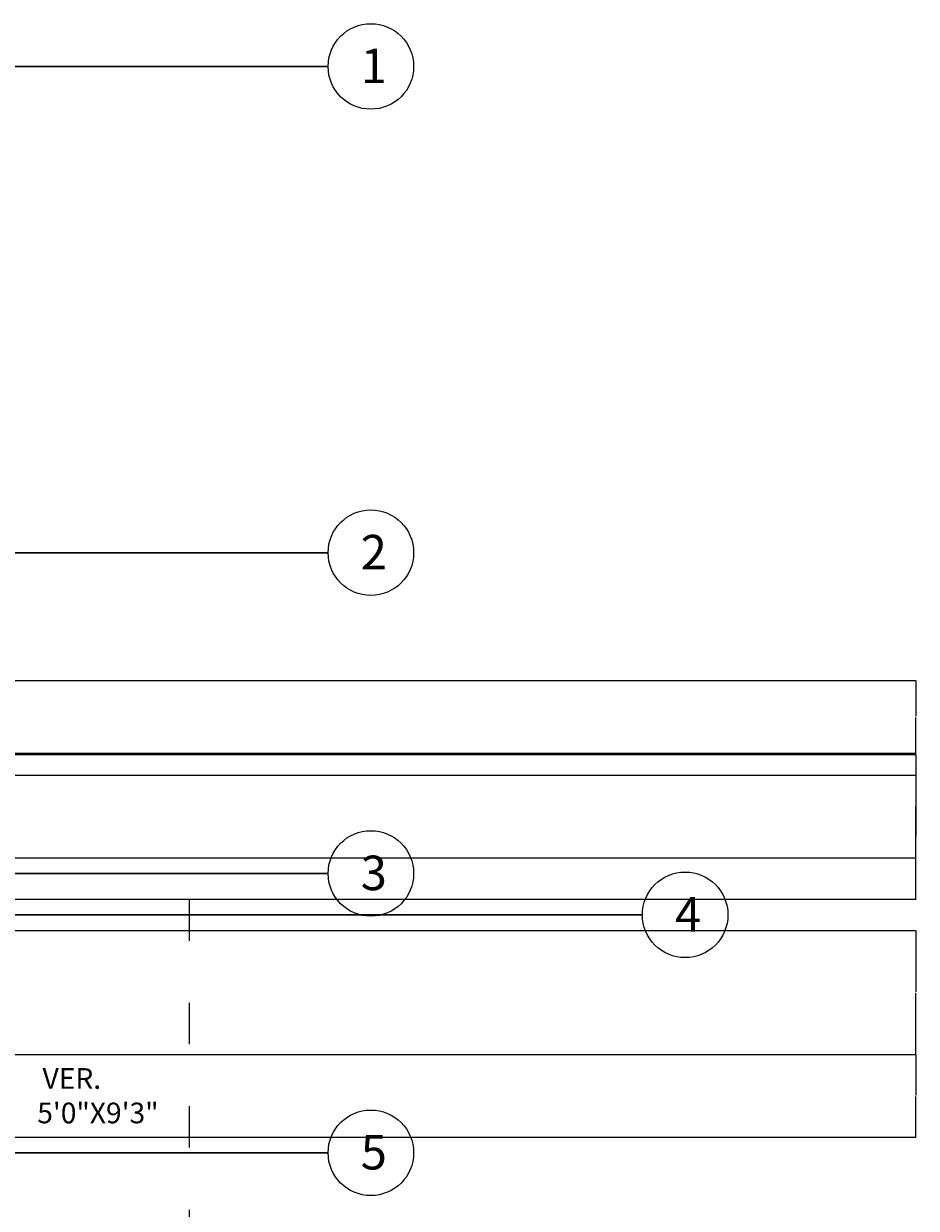
# Model space of a CAD drawing. Units: inches. Extents: x 5716 to 6907, y 12769 to 13594.
# Tile 17 of 17: x 6648 to 6907, y 13105 to 13448. Entities that reach past the tile are written whole.
import ezdxf

# ---------------------------------------------------------------- set-up
doc = ezdxf.new("R2010")
doc.units = ezdxf.units.IN
doc.linetypes.add('ACAD_ISO03W100', pattern=[30, 12, -18])
for name, color, linetype, lineweight in [('A-ANNO-DIMS', 2, 'Continuous', 18), ('A-AREA-IDEN', 7, 'Continuous', 18), ('A-FLOR-OVHD', 8, 'ACAD_ISO03W100', 18), ('A-GRID', 8, 'Continuous', 13), ('A-GRID-IDEN', 7, 'Continuous', 18)]:
    doc.layers.add(name, color=color, linetype=linetype, lineweight=lineweight)
doc.styles.get("Standard").update_dxf_attribs({"font": 'arial.ttf'})
doc.dimstyles.get("Standard").update_dxf_attribs({"dimtxt": 0.18, "dimasz": 0.18, "dimexe": 0.18, "dimexo": 0.0625, "dimgap": 0.09, "dimtad": 0, "dimtih": 1, "dimtoh": 1, "dimdec": 4, "dimzin": 0, "dimdsep": 46, "dimtxsty": 'Standard', "dimcen": 0.09, "dimadec": 0, "dimazin": 0, "dimtfac": 1, "dimtdec": 4, "dimtofl": 0, "dimtmove": 0, "dimatfit": 3, "dimfxl": 1, "dimtolj": 1, "dimtzin": 0, "dimarcsym": 0})

# ---------------------------------------------------------------- blocks, each defined once
blk = doc.blocks.new('*D58')
at = {"layer": 'A-ANNO-DIMS', "color": 0, "lineweight": -2, "transparency": 16777216}
for p, q in [((6736.67, 13435.65), (5716.04, 13435.65)), ((5716.22, 13435.47), (5716.22, 13365.33)), ((5716.22, 13294.83), (5716.22, 13364.97)), ((6736.67, 13294.65), (5716.04, 13294.65))]:
    blk.add_line(p, q, dxfattribs=at)
at = {"layer": 'A-ANNO-DIMS', "color": 0, "transparency": 16777216}
for points in [[(5716.19, 13435.47), (5716.25, 13435.47), (5716.22, 13435.65)], [(5716.19, 13294.83), (5716.25, 13294.83), (5716.22, 13294.65)]]:
    blk.add_solid(points, dxfattribs=at)
at = {"layer": 'Defpoints', "color": 0, "transparency": 16777216}
for p in [(6736.73, 13435.65), (5716.22, 13294.65), (6736.73, 13294.65)]:
    blk.add_point(p, dxfattribs=at)
at = {"layer": 'A-ANNO-DIMS', "color": 0, "transparency": 16777216, "insert": (5716.22, 13365.15), "char_height": 0.18, "attachment_point": 5}
blk.add_mtext('\\A1;141', dxfattribs=at)
blk = doc.blocks.new('*D59')
at = {"layer": 'A-ANNO-DIMS', "color": 0, "lineweight": -2, "transparency": 16777216}
for p, q in [((6736.67, 13294.65), (5716.04, 13294.65)), ((5716.22, 13294.47), (5716.22, 13248.33)), ((5716.22, 13201.83), (5716.22, 13247.97)), ((6736.67, 13201.65), (5716.04, 13201.65))]:
    blk.add_line(p, q, dxfattribs=at)
at = {"layer": 'A-ANNO-DIMS', "color": 0, "transparency": 16777216}
for points in [[(5716.19, 13294.47), (5716.25, 13294.47), (5716.22, 13294.65)], [(5716.19, 13201.83), (5716.25, 13201.83), (5716.22, 13201.65)]]:
    blk.add_solid(points, dxfattribs=at)
at = {"layer": 'Defpoints', "color": 0, "transparency": 16777216}
for p in [(6736.73, 13294.65), (5716.22, 13201.65), (6736.73, 13201.65)]:
    blk.add_point(p, dxfattribs=at)
at = {"layer": 'A-ANNO-DIMS', "color": 0, "transparency": 16777216, "insert": (5716.22, 13248.15), "char_height": 0.18, "attachment_point": 5}
blk.add_mtext('\\A1;93', dxfattribs=at)
blk = doc.blocks.new('*D60')
at = {"layer": 'A-ANNO-DIMS', "color": 0, "lineweight": -2, "transparency": 16777216}
for p, q in [((6736.67, 13201.65), (5716.04, 13201.65)), ((5716.22, 13201.47), (5716.22, 13195.83)), ((5716.22, 13189.83), (5716.22, 13195.47)), ((6827.78, 13189.65), (5716.04, 13189.65))]:
    blk.add_line(p, q, dxfattribs=at)
at = {"layer": 'A-ANNO-DIMS', "color": 0, "transparency": 16777216}
for points in [[(5716.19, 13201.47), (5716.25, 13201.47), (5716.22, 13201.65)], [(5716.19, 13189.83), (5716.25, 13189.83), (5716.22, 13189.65)]]:
    blk.add_solid(points, dxfattribs=at)
at = {"layer": 'Defpoints', "color": 0, "transparency": 16777216}
for p in [(6736.73, 13201.65), (5716.22, 13189.65), (6827.84, 13189.65)]:
    blk.add_point(p, dxfattribs=at)
at = {"layer": 'A-ANNO-DIMS', "color": 0, "transparency": 16777216, "insert": (5716.22, 13195.65), "char_height": 0.18, "attachment_point": 5}
blk.add_mtext('\\A1;12', dxfattribs=at)
blk = doc.blocks.new('*D61')
at = {"layer": 'A-ANNO-DIMS', "color": 0, "lineweight": -2, "transparency": 16777216}
for p, q in [((6827.78, 13189.65), (5716.04, 13189.65)), ((5716.22, 13189.47), (5716.22, 13155.33)), ((5716.22, 13120.83), (5716.22, 13154.97)), ((6736.67, 13120.65), (5716.04, 13120.65))]:
    blk.add_line(p, q, dxfattribs=at)
at = {"layer": 'A-ANNO-DIMS', "color": 0, "transparency": 16777216}
for points in [[(5716.19, 13189.47), (5716.25, 13189.47), (5716.22, 13189.65)], [(5716.19, 13120.83), (5716.25, 13120.83), (5716.22, 13120.65)]]:
    blk.add_solid(points, dxfattribs=at)
at = {"layer": 'Defpoints', "color": 0, "transparency": 16777216}
for p in [(6827.84, 13189.65), (5716.22, 13120.65), (6736.73, 13120.65)]:
    blk.add_point(p, dxfattribs=at)
at = {"layer": 'A-ANNO-DIMS', "color": 0, "transparency": 16777216, "insert": (5716.22, 13155.15), "char_height": 0.18, "attachment_point": 5}
blk.add_mtext('\\A1;69', dxfattribs=at)
blk = doc.blocks.new('*D62')
at = {"layer": 'A-ANNO-DIMS', "color": 0, "lineweight": -2, "transparency": 16777216}
for p, q in [((6736.67, 13120.65), (5716.04, 13120.65)), ((5716.22, 13120.47), (5716.22, 13100.33)), ((5716.22, 13079.83), (5716.22, 13099.97)), ((6736.67, 13079.65), (5716.04, 13079.65))]:
    blk.add_line(p, q, dxfattribs=at)
at = {"layer": 'A-ANNO-DIMS', "color": 0, "transparency": 16777216}
for points in [[(5716.19, 13120.47), (5716.25, 13120.47), (5716.22, 13120.65)], [(5716.19, 13079.83), (5716.25, 13079.83), (5716.22, 13079.65)]]:
    blk.add_solid(points, dxfattribs=at)
at = {"layer": 'Defpoints', "color": 0, "transparency": 16777216}
for p in [(6736.73, 13120.65), (5716.22, 13079.65), (6736.73, 13079.65)]:
    blk.add_point(p, dxfattribs=at)
at = {"layer": 'A-ANNO-DIMS', "color": 0, "transparency": 16777216, "insert": (5716.22, 13100.15), "char_height": 0.18, "attachment_point": 5}
blk.add_mtext('\\A1;41', dxfattribs=at)
blk = doc.blocks.new('*D69')
at = {"layer": 'A-ANNO-DIMS', "color": 0, "lineweight": -2, "transparency": 16777216}
for p, q in [((5828.09, 13149.15), (6907.26, 13149.15)), ((6907.08, 13148.97), (6907.08, 13137.33)), ((6907.08, 13125.33), (6907.08, 13136.97)), ((5828.09, 13125.15), (6907.26, 13125.15))]:
    blk.add_line(p, q, dxfattribs=at)
at = {"layer": 'A-ANNO-DIMS', "color": 0, "transparency": 16777216}
for points in [[(6907.05, 13148.97), (6907.11, 13148.97), (6907.08, 13149.15)], [(6907.05, 13125.33), (6907.11, 13125.33), (6907.08, 13125.15)]]:
    blk.add_solid(points, dxfattribs=at)
at = {"layer": 'Defpoints', "color": 0, "transparency": 16777216}
for p in [(5828.02, 13149.15), (6907.08, 13149.15), (5828.02, 13125.15)]:
    blk.add_point(p, dxfattribs=at)
at = {"layer": 'A-ANNO-DIMS', "color": 0, "transparency": 16777216, "insert": (6907.08, 13137.15), "char_height": 0.18, "attachment_point": 5}
blk.add_mtext('\\A1;24', dxfattribs=at)
blk = doc.blocks.new('*D70')
at = {"layer": 'A-ANNO-DIMS', "color": 0, "lineweight": -2, "transparency": 16777216}
for p, q in [((5828.09, 13236.15), (6907.26, 13236.15)), ((6907.08, 13235.97), (6907.08, 13221.33)), ((6907.08, 13206.33), (6907.08, 13220.97)), ((5828.09, 13206.15), (6907.26, 13206.15))]:
    blk.add_line(p, q, dxfattribs=at)
at = {"layer": 'A-ANNO-DIMS', "color": 0, "transparency": 16777216}
for points in [[(6907.05, 13235.97), (6907.11, 13235.97), (6907.08, 13236.15)], [(6907.05, 13206.33), (6907.11, 13206.33), (6907.08, 13206.15)]]:
    blk.add_solid(points, dxfattribs=at)
at = {"layer": 'Defpoints', "color": 0, "transparency": 16777216}
for p in [(5828.02, 13236.15), (6907.08, 13236.15), (5828.02, 13206.15)]:
    blk.add_point(p, dxfattribs=at)
at = {"layer": 'A-ANNO-DIMS', "color": 0, "transparency": 16777216, "insert": (6907.08, 13221.15), "char_height": 0.18, "attachment_point": 5}
blk.add_mtext('\\A1;30', dxfattribs=at)
blk = doc.blocks.new('*D71')
at = {"layer": 'A-ANNO-DIMS', "color": 0, "lineweight": -2, "transparency": 16777216}
for p, q in [((6188.09, 13230.15), (6907.26, 13230.15)), ((6907.08, 13229.97), (6907.08, 13212.33)), ((6907.08, 13194.33), (6907.08, 13211.97)), ((6179.09, 13194.15), (6907.26, 13194.15))]:
    blk.add_line(p, q, dxfattribs=at)
at = {"layer": 'A-ANNO-DIMS', "color": 0, "transparency": 16777216}
for points in [[(6907.05, 13229.97), (6907.11, 13229.97), (6907.08, 13230.15)], [(6907.05, 13194.33), (6907.11, 13194.33), (6907.08, 13194.15)]]:
    blk.add_solid(points, dxfattribs=at)
at = {"layer": 'Defpoints', "color": 0, "transparency": 16777216}
for p in [(6188.02, 13230.15), (6907.08, 13230.15), (6179.02, 13194.15)]:
    blk.add_point(p, dxfattribs=at)
at = {"layer": 'A-ANNO-DIMS', "color": 0, "transparency": 16777216, "insert": (6907.08, 13212.15), "char_height": 0.18, "attachment_point": 5}
blk.add_mtext('\\A1;36', dxfattribs=at)
blk = doc.blocks.new('*D74')
at = {"layer": 'A-ANNO-DIMS', "color": 0, "lineweight": -2, "transparency": 16777216}
for p, q in [((6188.09, 13185.15), (6907.26, 13185.15)), ((6907.08, 13184.97), (6907.08, 13167.33)), ((6907.08, 13149.33), (6907.08, 13166.97)), ((6188.09, 13149.15), (6907.26, 13149.15))]:
    blk.add_line(p, q, dxfattribs=at)
at = {"layer": 'A-ANNO-DIMS', "color": 0, "transparency": 16777216}
for points in [[(6907.05, 13184.97), (6907.11, 13184.97), (6907.08, 13185.15)], [(6907.05, 13149.33), (6907.11, 13149.33), (6907.08, 13149.15)]]:
    blk.add_solid(points, dxfattribs=at)
at = {"layer": 'Defpoints', "color": 0, "transparency": 16777216}
for p in [(6188.02, 13185.15), (6907.08, 13185.15), (6188.02, 13149.15)]:
    blk.add_point(p, dxfattribs=at)
at = {"layer": 'A-ANNO-DIMS', "color": 0, "transparency": 16777216, "insert": (6907.08, 13167.15), "char_height": 0.18, "attachment_point": 5}
blk.add_mtext('\\A1;36', dxfattribs=at)
blk = doc.blocks.new('*D76')
at = {"layer": 'A-ANNO-DIMS', "color": 0, "lineweight": -2, "transparency": 16777216}
for p, q in [((5830.73, 13257.56), (6907.26, 13257.56)), ((6907.08, 13257.38), (6907.08, 13247.24)), ((6907.08, 13236.74), (6907.08, 13246.88)), ((5830.73, 13236.56), (6907.26, 13236.56))]:
    blk.add_line(p, q, dxfattribs=at)
at = {"layer": 'A-ANNO-DIMS', "color": 0, "transparency": 16777216}
for points in [[(6907.05, 13257.38), (6907.11, 13257.38), (6907.08, 13257.56)], [(6907.05, 13236.74), (6907.11, 13236.74), (6907.08, 13236.56)]]:
    blk.add_solid(points, dxfattribs=at)
at = {"layer": 'Defpoints', "color": 0, "transparency": 16777216}
for p in [(5830.67, 13257.56), (5830.67, 13236.56), (6907.08, 13236.56)]:
    blk.add_point(p, dxfattribs=at)
at = {"layer": 'A-ANNO-DIMS', "color": 0, "transparency": 16777216, "insert": (6907.08, 13247.06), "char_height": 0.18, "attachment_point": 5}
blk.add_mtext('\\A1;21', dxfattribs=at)

msp = doc.modelspace()

# ---------------------------------------------------------------- linework, layer by layer
at = {"layer": 'A-FLOR-OVHD'}
for p, q in [((6636.41, 13194.15), (6696.41, 13194.15)), ((6696.41, 13194.15), (6696.41, 13075.15))]:
    msp.add_line(p, q, dxfattribs=at)
at = {"layer": 'A-GRID'}
for p, q in [((6267.41, 13435.65), (6736.73, 13435.65)), ((6267.41, 13294.65), (6736.73, 13294.65)), ((6267.41, 13201.65), (6736.73, 13201.65)), ((6267.41, 13189.65), (6827.84, 13189.65)), ((6267.41, 13120.65), (6736.73, 13120.65))]:
    msp.add_line(p, q, dxfattribs=at)
at = {"layer": 'A-GRID-IDEN'}
for centre in [(6749.12, 13435.65), (6749.12, 13294.65), (6749.12, 13201.65), (6840.24, 13189.65), (6749.12, 13120.65)]:
    msp.add_circle(centre, 12.4, dxfattribs=at)

# ---------------------------------------------------------------- texts
at = {"layer": 'A-AREA-IDEN', "insert": (6652.38, 13145.2), "char_height": 2.5, "attachment_point": 1}
msp.add_mtext_dynamic_manual_height_columns('  {\\H2.4x;VER.\\P5\'0"X9\'3"}', width=37.6647, gutter_width=12.5, heights=[0], dxfattribs=at)
at = {"layer": 'A-GRID-IDEN', "char_height": 10, "attachment_point": 1}
for s, insert in [('1', (6746.18, 13440.81)), ('2', (6746.18, 13299.81)), ('3', (6746.18, 13206.81)), ('4', (6837.29, 13194.81)), ('5', (6746.18, 13125.81))]:
    msp.add_mtext_dynamic_manual_height_columns(s, width=121.9272, gutter_width=12.5, heights=[0], dxfattribs=dict(at, insert=insert))

# ---------------------------------------------------------------- dimensions: what is measured, and where the dimension line sits
at = {"layer": 'A-ANNO-DIMS'}
for base, p1, p2, picture, middle in [((5716.22, 13294.65), (6736.73, 13435.65), (6736.73, 13294.65), '*D58', (5716.22, 13365.15)), ((5716.22, 13201.65), (6736.73, 13294.65), (6736.73, 13201.65), '*D59', (5716.22, 13248.15)), ((6907.08, 13236.56), (5830.67, 13257.56), (5830.67, 13236.56), '*D76', (6907.08, 13247.06)), ((6907.08, 13236.15), (5828.02, 13206.15), (5828.02, 13236.15), '*D70', (6907.08, 13221.15)), ((6907.08, 13230.15), (6179.02, 13194.15), (6188.02, 13230.15), '*D71', (6907.08, 13212.15)), ((5716.22, 13189.65), (6736.73, 13201.65), (6827.84, 13189.65), '*D60', (5716.22, 13195.65)), ((5716.22, 13120.65), (6827.84, 13189.65), (6736.73, 13120.65), '*D61', (5716.22, 13155.15)), ((6907.08, 13185.15), (6188.02, 13149.15), (6188.02, 13185.15), '*D74', (6907.08, 13167.15)), ((6907.08, 13149.15), (5828.02, 13125.15), (5828.02, 13149.15), '*D69', (6907.08, 13137.15)), ((5716.22, 13079.65), (6736.73, 13120.65), (6736.73, 13079.65), '*D62', (5716.22, 13100.15))]:
    dim = msp.add_linear_dim(base=base, p1=p1, p2=p2, angle=90, dimstyle='Standard', override={"dimdec": 0, "dimlfac": 1, "dimrnd": 0, "dimzin": 0, "dimdsep": 46, "dimlunit": 2}, dxfattribs=at)
    dim.commit()
    dim.dimension.update_dxf_attribs({"geometry": picture, "text_midpoint": middle})

doc.saveas('drawing.dxf')
